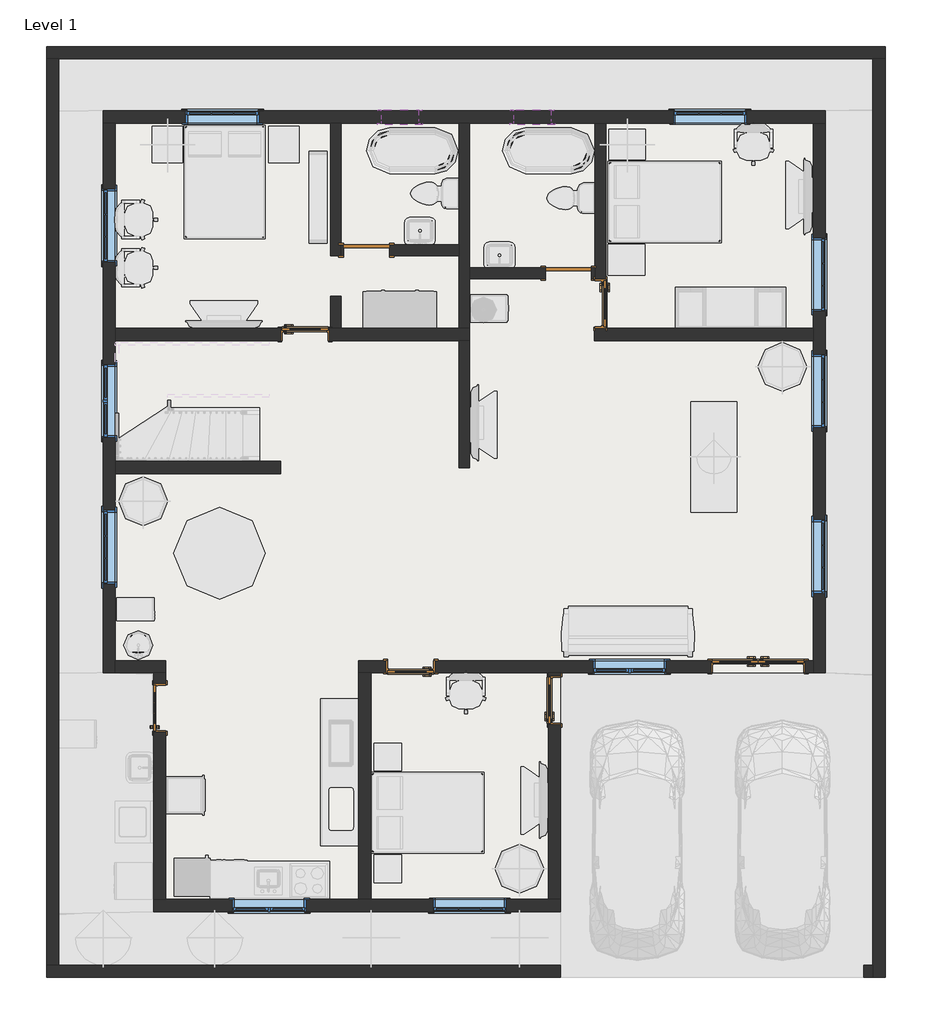
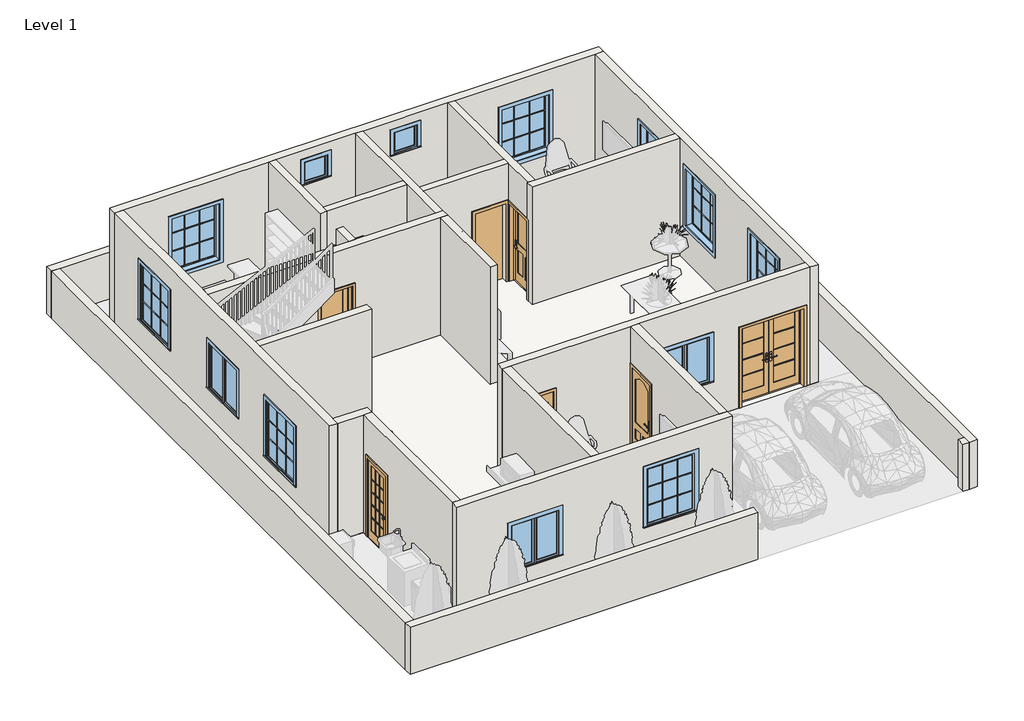
# One storey, part 1 of 3: 24 walls, 13 windows, 8 doors, 1 slab.
"""IFC4 building model written with IfcOpenShell, lengths in millimetres."""

from ifc_helpers import new_model, si_unit, frame, origin, origin_with_axes, place, context, project, spatial, polyline, outline, extrude, faceted_brep, transform, mapped, element, save
from components import door_41326d50, door_7e6851c9, door_3dfc5bb7, door_b03bd389, door_fe2643c7, door_ebd1a24e, door_41c6c2d7, window_cfa1ffdd, window_0862ab64, window_e41d21a6

model = new_model("IFC4")

# Units and contexts
model_context = context("Model", 3, world=origin())
ifc_project = project(units=[si_unit("LENGTHUNIT", "METRE", prefix="MILLI")], contexts=[model_context])

# Site, building, storey
site = spatial("IfcSite", under=ifc_project)
building = spatial("IfcBuilding", under=site)
storey = spatial("IfcBuildingStorey", under=building, Name="Level 1", Elevation=0.0)

# Doors
placement = place(None, origin())
door_shape = door_41326d50(model_context)
element("IfcDoor", 1, ObjectType="30\" x 80\"", at=placement, inside=storey, context=model_context, shape_type="MappedRepresentation", body=[
    mapped(door_shape, transform((-7358.6481534, 4188.5162111, 0.0), x_axis=(0.0, -1.0, 0.0), y_axis=(1.0, 0.0, 0.0), z_axis=(0.0, 0.0, 1.0))),
])
element("IfcDoor", 2, ObjectType="30\" x 80\"", at=placement, inside=storey, context=model_context, shape_type="MappedRepresentation", body=[
    mapped(door_shape, transform((-9743.0731534, 4744.1412111, 0.0), x_axis=(1.0, 0.0, 0.0), y_axis=(0.0, 1.0, 0.0), z_axis=(0.0, 0.0, 1.0))),
])
door_2_shape = door_7e6851c9(model_context)
element("IfcDoor", 3, ObjectType="30\" x 80\"", at=placement, inside=storey, context=model_context, shape_type="MappedRepresentation", body=[
    mapped(door_2_shape, transform((-11495.6731534, 10262.2912111, 0.0), x_axis=(-1.0, 0.0, 0.0), y_axis=(0.0, -1.0, 0.0), z_axis=(0.0, 0.0, 1.0))),
])
door_3_shape = door_3dfc5bb7(model_context)
element("IfcDoor", 4, ObjectType="30\" x 80\"", at=placement, inside=storey, context=model_context, shape_type="MappedRepresentation", body=[
    mapped(door_3_shape, transform((-6590.2981534, 10767.1162111, 0.0), x_axis=(0.0, 1.0, 0.0), y_axis=(-1.0, 0.0, 0.0), z_axis=(0.0, 0.0, 1.0))),
])
door_4_shape = door_b03bd389(model_context)
element("IfcDoor", 5, ObjectType="Door-Exterior-Double-Full Glass-Wood_Clad : 60\" x 80\"", at=placement, inside=storey, context=model_context, shape_type="MappedRepresentation", body=[
    mapped(door_4_shape, transform((-3977.2731534, 4750.4912111, 0.0), x_axis=(1.0, 0.0, 0.0), y_axis=(0.0, 1.0, 0.0), z_axis=(0.0, 0.0, 1.0))),
])
door_5_shape = door_fe2643c7(model_context)
element("IfcDoor", 6, ObjectType="Door-Interior-Single-Full Glass-Wood : 30\" x 80\"", at=placement, inside=storey, context=model_context, shape_type="MappedRepresentation", body=[
    mapped(door_5_shape, transform((-13911.8481534, 4061.5162111, 0.0), x_axis=(0.0, 1.0, 0.0), y_axis=(-1.0, 0.0, 0.0), z_axis=(0.0, 0.0, 1.0))),
])
door_6_shape = door_ebd1a24e(model_context)
element("IfcDoor", 7, ObjectType="Single-Flush : 30\" x 80\"", at=placement, inside=storey, context=model_context, shape_type="MappedRepresentation", body=[
    mapped(door_6_shape, transform((-10479.6731534, 11656.1162111, 0.0), x_axis=(-1.0, 0.0, 0.0), y_axis=(0.0, -1.0, 0.0), z_axis=(0.0, 0.0, 1.0))),
])
door_7_shape = door_41c6c2d7(model_context)
element("IfcDoor", 8, ObjectType="Single-Flush : 30\" x 80\"", at=placement, inside=storey, context=model_context, shape_type="MappedRepresentation", body=[
    mapped(door_7_shape, transform((-7126.8731534, 11275.1162111, 0.0), x_axis=(1.0, 0.0, 0.0), y_axis=(0.0, 1.0, 0.0), z_axis=(0.0, 0.0, 1.0))),
])

# Slab
element("IfcSlab", 9, at=placement, inside=storey, context=model_context, shape_type="SweptSolid", body=[
    extrude(outline(polyline([(-2859.6731534, 13967.5162111), (-2859.6731534, 4645.7162111), (-7253.8731534, 4645.7162111), (-7253.8731534, 683.3162111), (-14010.2731534, 683.3162111), (-14010.2731534, 4645.7162111), (-14848.4731534, 4645.7162111), (-14848.4731534, 13967.5162111), (-2859.6731534, 13967.5162111)])), frame((0.0, 0.0, -323.85), z_axis=(0.0, 0.0, 1.0), x_axis=(1.0, 0.0, 0.0)), (0.0, 0.0, 1.0), 323.85),
])

# Walls
element("IfcWall", 10, ObjectType="Generic - 8\"", at=placement, inside=storey, context=model_context, shape_type="SweptSolid", body=[
    extrude(outline(polyline([(-2224.6731534, -205.6837889), (-2072.2731534, -205.6837889), (-2072.2731534, -408.8837889), (-2224.6731534, -408.8837889), (-2224.6731534, -205.6837889)])), origin_with_axes(), (0.0, 0.0, 1.0), 1219.2),
])
element("IfcWall", 11, ObjectType="Generic - 8\"", at=placement, inside=storey, context=model_context, shape_type="Brep", body=[
    faceted_brep([(-14848.4731534, 13764.3162111, 0.0), (-14848.4731534, 4645.7162111, 0.0), (-14848.4731534, 4645.7162111, 3048.0), (-14848.4731534, 13764.3162111, 3048.0), (-14848.4731534, 7338.1162111, 2133.6), (-14848.4731534, 6118.9162111, 2133.6), (-14848.4731534, 6118.9162111, 609.6), (-14848.4731534, 7338.1162111, 609.6), (-14848.4731534, 12672.1162111, 2438.4), (-14848.4731534, 11452.9162111, 2438.4), (-14848.4731534, 11452.9162111, 914.4), (-14848.4731534, 12672.1162111, 914.4), (-14848.4731534, 9763.8162111, 2133.6), (-14848.4731534, 8544.6162111, 2133.6), (-14848.4731534, 8544.6162111, 914.4), (-14848.4731534, 9763.8162111, 914.4), (-14645.2731534, 13764.3162111, 0.0), (-14645.2731534, 13764.3162111, 3048.0), (-14645.2731534, 10360.7162111, 3048.0), (-14645.2731534, 10157.5162111, 3048.0), (-14645.2731534, 8150.9162111, 3048.0), (-14645.2731534, 7947.7162111, 3048.0), (-14645.2731534, 4848.9162111, 3048.0), (-14645.2731534, 4645.7162111, 3048.0), (-14645.2731534, 4645.7162111, 0.0), (-14645.2731534, 4848.9162111, 0.0), (-14645.2731534, 7947.7162111, 0.0), (-14645.2731534, 8150.9162111, 0.0), (-14645.2731534, 10157.5162111, 0.0), (-14645.2731534, 10360.7162111, 0.0), (-14645.2731534, 7338.1162111, 2133.6), (-14645.2731534, 7338.1162111, 609.6), (-14645.2731534, 6118.9162111, 609.6), (-14645.2731534, 6118.9162111, 2133.6), (-14645.2731534, 12672.1162111, 2438.4), (-14645.2731534, 12672.1162111, 914.4), (-14645.2731534, 11452.9162111, 914.4), (-14645.2731534, 11452.9162111, 2438.4), (-14645.2731534, 9763.8162111, 2133.6), (-14645.2731534, 9763.8162111, 914.4), (-14645.2731534, 8544.6162111, 914.4), (-14645.2731534, 8544.6162111, 2133.6)], [[[0, 1, 2, 3], [4, 5, 6, 7], [8, 9, 10, 11], [12, 13, 14, 15]], [[16, 17, 18, 19, 20, 21, 22, 23, 24, 25, 26, 27, 28, 29], [30, 31, 32, 33], [34, 35, 36, 37], [38, 39, 40, 41]], [[1, 0, 16, 29, 28, 27, 26, 25, 24]], [[3, 2, 23, 22, 21, 20, 19, 18, 17]], [[0, 3, 17, 16]], [[2, 1, 24, 23]], [[31, 30, 4, 7]], [[32, 31, 7, 6]], [[33, 32, 6, 5]], [[30, 33, 5, 4]], [[35, 34, 8, 11]], [[36, 35, 11, 10]], [[37, 36, 10, 9]], [[34, 37, 9, 8]], [[39, 38, 12, 15]], [[40, 39, 15, 14]], [[41, 40, 14, 13]], [[38, 41, 13, 12]]]),
])
element("IfcWall", 12, ObjectType="Generic - 8\"", at=placement, inside=storey, context=model_context, shape_type="Brep", body=[
    faceted_brep([(-3062.8731534, 13764.3162111, 0.0), (-3062.8731534, 10360.7162111, 0.0), (-3062.8731534, 10157.5162111, 0.0), (-3062.8731534, 4848.9162111, 0.0), (-3062.8731534, 4645.7162111, 0.0), (-3062.8731534, 4645.7162111, 3048.0), (-3062.8731534, 4848.9162111, 3048.0), (-3062.8731534, 10157.5162111, 3048.0), (-3062.8731534, 10360.7162111, 3048.0), (-3062.8731534, 13764.3162111, 3048.0), (-3062.8731534, 10640.1162111, 2438.4), (-3062.8731534, 10640.1162111, 914.4), (-3062.8731534, 11859.3162111, 914.4), (-3062.8731534, 11859.3162111, 2438.4), (-3062.8731534, 8709.7162111, 2438.4), (-3062.8731534, 8709.7162111, 914.4), (-3062.8731534, 9928.9162111, 914.4), (-3062.8731534, 9928.9162111, 2438.4), (-3062.8731534, 5966.5162111, 2438.4), (-3062.8731534, 5966.5162111, 914.4), (-3062.8731534, 7185.7162111, 914.4), (-3062.8731534, 7185.7162111, 2438.4), (-2859.6731534, 13764.3162111, 0.0), (-2859.6731534, 13764.3162111, 3048.0), (-2859.6731534, 4645.7162111, 3048.0), (-2859.6731534, 4645.7162111, 0.0), (-2859.6731534, 10640.1162111, 2438.4), (-2859.6731534, 11859.3162111, 2438.4), (-2859.6731534, 11859.3162111, 914.4), (-2859.6731534, 10640.1162111, 914.4), (-2859.6731534, 8709.7162111, 2438.4), (-2859.6731534, 9928.9162111, 2438.4), (-2859.6731534, 9928.9162111, 914.4), (-2859.6731534, 8709.7162111, 914.4), (-2859.6731534, 5966.5162111, 2438.4), (-2859.6731534, 7185.7162111, 2438.4), (-2859.6731534, 7185.7162111, 914.4), (-2859.6731534, 5966.5162111, 914.4)], [[[0, 1, 2, 3, 4, 5, 6, 7, 8, 9], [10, 11, 12, 13], [14, 15, 16, 17], [18, 19, 20, 21]], [[22, 23, 24, 25], [26, 27, 28, 29], [30, 31, 32, 33], [34, 35, 36, 37]], [[4, 3, 2, 1, 0, 22, 25]], [[9, 8, 7, 6, 5, 24, 23]], [[0, 9, 23, 22]], [[5, 4, 25, 24]], [[11, 10, 26, 29]], [[12, 11, 29, 28]], [[13, 12, 28, 27]], [[10, 13, 27, 26]], [[15, 14, 30, 33]], [[16, 15, 33, 32]], [[17, 16, 32, 31]], [[14, 17, 31, 30]], [[19, 18, 34, 37]], [[20, 19, 37, 36]], [[21, 20, 36, 35]], [[18, 21, 35, 34]]]),
])
element("IfcWall", 13, ObjectType="Generic - 8\"", at=placement, inside=storey, context=model_context, shape_type="Brep", body=[
    faceted_brep([(-2859.6731534, 13967.5162111, 0.0), (-14848.4731534, 13967.5162111, 0.0), (-14848.4731534, 13967.5162111, 3048.0), (-2859.6731534, 13967.5162111, 3048.0), (-12257.6731534, 13967.5162111, 2438.4), (-13476.8731534, 13967.5162111, 2438.4), (-13476.8731534, 13967.5162111, 914.4), (-12257.6731534, 13967.5162111, 914.4), (-4167.7731534, 13967.5162111, 2438.4), (-5386.9731534, 13967.5162111, 2438.4), (-5386.9731534, 13967.5162111, 914.4), (-4167.7731534, 13967.5162111, 914.4), (-10225.6731534, 13967.5162111, 2768.6), (-10225.6731534, 13967.5162111, 2159.0), (-9616.0731534, 13967.5162111, 2159.0), (-9616.0731534, 13967.5162111, 2768.6), (-8028.5731534, 13967.5162111, 2768.6), (-8028.5731534, 13967.5162111, 2159.0), (-7418.9731534, 13967.5162111, 2159.0), (-7418.9731534, 13967.5162111, 2768.6), (-2859.6731534, 13764.3162111, 0.0), (-2859.6731534, 13764.3162111, 3048.0), (-3062.8731534, 13764.3162111, 3048.0), (-6504.5731534, 13764.3162111, 3048.0), (-6682.3731534, 13764.3162111, 3048.0), (-8765.1731534, 13764.3162111, 3048.0), (-8942.9731534, 13764.3162111, 3048.0), (-10898.7731534, 13764.3162111, 3048.0), (-11076.5731534, 13764.3162111, 3048.0), (-14645.2731534, 13764.3162111, 3048.0), (-14848.4731534, 13764.3162111, 3048.0), (-14848.4731534, 13764.3162111, 0.0), (-14645.2731534, 13764.3162111, 0.0), (-11076.5731534, 13764.3162111, 0.0), (-10898.7731534, 13764.3162111, 0.0), (-8942.9731534, 13764.3162111, 0.0), (-8765.1731534, 13764.3162111, 0.0), (-6682.3731534, 13764.3162111, 0.0), (-6504.5731534, 13764.3162111, 0.0), (-3062.8731534, 13764.3162111, 0.0), (-12257.6731534, 13764.3162111, 2438.4), (-12257.6731534, 13764.3162111, 914.4), (-13476.8731534, 13764.3162111, 914.4), (-13476.8731534, 13764.3162111, 2438.4), (-4167.7731534, 13764.3162111, 2438.4), (-4167.7731534, 13764.3162111, 914.4), (-5386.9731534, 13764.3162111, 914.4), (-5386.9731534, 13764.3162111, 2438.4), (-10225.6731534, 13764.3162111, 2768.6), (-9616.0731534, 13764.3162111, 2768.6), (-9616.0731534, 13764.3162111, 2159.0), (-10225.6731534, 13764.3162111, 2159.0), (-8028.5731534, 13764.3162111, 2768.6), (-7418.9731534, 13764.3162111, 2768.6), (-7418.9731534, 13764.3162111, 2159.0), (-8028.5731534, 13764.3162111, 2159.0)], [[[0, 1, 2, 3], [4, 5, 6, 7], [8, 9, 10, 11], [12, 13, 14, 15], [16, 17, 18, 19]], [[20, 21, 22, 23, 24, 25, 26, 27, 28, 29, 30, 31, 32, 33, 34, 35, 36, 37, 38, 39], [40, 41, 42, 43], [44, 45, 46, 47], [48, 49, 50, 51], [52, 53, 54, 55]], [[1, 0, 20, 39, 38, 37, 36, 35, 34, 33, 32, 31]], [[3, 2, 30, 29, 28, 27, 26, 25, 24, 23, 22, 21]], [[2, 1, 31, 30]], [[0, 3, 21, 20]], [[41, 40, 4, 7]], [[42, 41, 7, 6]], [[43, 42, 6, 5]], [[40, 43, 5, 4]], [[45, 44, 8, 11]], [[46, 45, 11, 10]], [[47, 46, 10, 9]], [[44, 47, 9, 8]], [[13, 12, 48, 51]], [[14, 13, 51, 50]], [[15, 14, 50, 49]], [[12, 15, 49, 48]], [[17, 16, 52, 55]], [[18, 17, 55, 54]], [[19, 18, 54, 53]], [[16, 19, 53, 52]]]),
])
element("IfcWall", 14, ObjectType="Generic - 8\"", at=placement, inside=storey, context=model_context, shape_type="Brep", body=[
    faceted_brep([(-14645.2731534, 4645.7162111, 0.0), (-14010.2731534, 4645.7162111, 0.0), (-13807.0731534, 4645.7162111, 0.0), (-13807.0731534, 4645.7162111, 3048.0), (-14010.2731534, 4645.7162111, 3048.0), (-14645.2731534, 4645.7162111, 3048.0), (-14645.2731534, 4848.9162111, 0.0), (-14645.2731534, 4848.9162111, 3048.0), (-13807.0731534, 4848.9162111, 3048.0), (-13807.0731534, 4848.9162111, 0.0)], [[[0, 1, 2, 3, 4, 5]], [[6, 7, 8, 9]], [[2, 1, 0, 6, 9]], [[3, 2, 9, 8]], [[5, 4, 3, 8, 7]], [[0, 5, 7, 6]]]),
])
element("IfcWall", 15, ObjectType="Generic - 8\"", at=placement, inside=storey, context=model_context, shape_type="SweptSolid", body=[
    extrude(outline(polyline([(-10606.6731534, 886.5162111), (-10606.6731534, 4645.7162111), (-10403.4731534, 4645.7162111), (-10403.4731534, 886.5162111), (-10606.6731534, 886.5162111)])), origin_with_axes(), (0.0, 0.0, 1.0), 3048.0),
])
element("IfcWall", 16, ObjectType="Generic - 8\"", at=placement, inside=storey, context=model_context, shape_type="SweptSolid", body=[
    extrude(outline(polyline([(886.5162111, 3048.0), (4645.7162111, 3048.0), (4645.7162111, 0.0), (4467.9162111, 0.0), (4467.9162111, 2057.4), (3655.1162111, 2057.4), (3655.1162111, 0.0), (886.5162111, 0.0), (886.5162111, 3048.0)])), frame((-14010.2731534, 0.0, 0.0), z_axis=(1.0, 0.0, 0.0), x_axis=(0.0, 1.0, 0.0)), (0.0, 0.0, 1.0), 203.2),
])
element("IfcWall", 17, ObjectType="Generic - 8\"", at=placement, inside=storey, context=model_context, shape_type="Brep", body=[
    faceted_brep([(-14010.2731534, 683.3162111, 0.0), (-7253.8731534, 683.3162111, 0.0), (-7253.8731534, 683.3162111, 3048.0), (-14010.2731534, 683.3162111, 3048.0), (-9374.7731534, 683.3162111, 2438.4), (-8155.5731534, 683.3162111, 2438.4), (-8155.5731534, 683.3162111, 914.4), (-9374.7731534, 683.3162111, 914.4), (-12702.1731534, 683.3162111, 2133.6), (-11482.9731534, 683.3162111, 2133.6), (-11482.9731534, 683.3162111, 914.4), (-12702.1731534, 683.3162111, 914.4), (-14010.2731534, 886.5162111, 0.0), (-14010.2731534, 886.5162111, 3048.0), (-13807.0731534, 886.5162111, 3048.0), (-10606.6731534, 886.5162111, 3048.0), (-10403.4731534, 886.5162111, 3048.0), (-7457.0731534, 886.5162111, 3048.0), (-7253.8731534, 886.5162111, 3048.0), (-7253.8731534, 886.5162111, 0.0), (-7457.0731534, 886.5162111, 0.0), (-10403.4731534, 886.5162111, 0.0), (-10606.6731534, 886.5162111, 0.0), (-13807.0731534, 886.5162111, 0.0), (-9374.7731534, 886.5162111, 2438.4), (-9374.7731534, 886.5162111, 914.4), (-8155.5731534, 886.5162111, 914.4), (-8155.5731534, 886.5162111, 2438.4), (-12702.1731534, 886.5162111, 2133.6), (-12702.1731534, 886.5162111, 914.4), (-11482.9731534, 886.5162111, 914.4), (-11482.9731534, 886.5162111, 2133.6)], [[[0, 1, 2, 3], [4, 5, 6, 7], [8, 9, 10, 11]], [[12, 13, 14, 15, 16, 17, 18, 19, 20, 21, 22, 23], [24, 25, 26, 27], [28, 29, 30, 31]], [[1, 0, 12, 23, 22, 21, 20, 19]], [[3, 2, 18, 17, 16, 15, 14, 13]], [[0, 3, 13, 12]], [[2, 1, 19, 18]], [[25, 24, 4, 7]], [[26, 25, 7, 6]], [[27, 26, 6, 5]], [[24, 27, 5, 4]], [[29, 28, 8, 11]], [[30, 29, 11, 10]], [[31, 30, 10, 9]], [[28, 31, 9, 8]]]),
])
element("IfcWall", 18, ObjectType="Generic - 8\"", at=placement, inside=storey, context=model_context, shape_type="SweptSolid", body=[
    extrude(outline(polyline([(886.5162111, 3048.0), (4645.7162111, 3048.0), (4645.7162111, 0.0), (4594.9162111, 0.0), (4594.9162111, 2057.4), (3782.1162111, 2057.4), (3782.1162111, 0.0), (886.5162111, 0.0), (886.5162111, 3048.0)])), frame((-7457.0731534, 0.0, 0.0), z_axis=(1.0, 0.0, 0.0), x_axis=(0.0, 1.0, 0.0)), (0.0, 0.0, 1.0), 203.2),
])
element("IfcWall", 19, ObjectType="Generic - 8\"", at=placement, inside=storey, context=model_context, shape_type="Brep", body=[
    faceted_brep([(-8765.1731534, 10157.5162111, 3048.0), (-8942.9731534, 10157.5162111, 3048.0), (-14645.2731534, 10157.5162111, 3048.0), (-14645.2731534, 10157.5162111, 0.0), (-11902.0731534, 10157.5162111, 0.0), (-11902.0731534, 10157.5162111, 2057.4), (-11089.2731534, 10157.5162111, 2057.4), (-11089.2731534, 10157.5162111, 0.0), (-8942.9731534, 10157.5162111, 0.0), (-8765.1731534, 10157.5162111, 0.0), (-14645.2731534, 10360.7162111, 3048.0), (-11076.5731534, 10360.7162111, 3048.0), (-10898.7731534, 10360.7162111, 3048.0), (-8942.9731534, 10360.7162111, 3048.0), (-8765.1731534, 10360.7162111, 3048.0), (-8765.1731534, 10360.7162111, 0.0), (-8942.9731534, 10360.7162111, 0.0), (-10898.7731534, 10360.7162111, 0.0), (-11076.5731534, 10360.7162111, 0.0), (-11089.2731534, 10360.7162111, 0.0), (-11089.2731534, 10360.7162111, 2057.4), (-11902.0731534, 10360.7162111, 2057.4), (-11902.0731534, 10360.7162111, 0.0), (-14645.2731534, 10360.7162111, 0.0)], [[[0, 1, 2, 3, 4, 5, 6, 7, 8, 9]], [[10, 11, 12, 13, 14, 15, 16, 17, 18, 19, 20, 21, 22, 23]], [[3, 23, 22, 4]], [[15, 9, 8, 7, 19, 18, 17, 16]], [[2, 1, 0, 14, 13, 12, 11, 10]], [[3, 2, 10, 23]], [[0, 9, 15, 14]], [[21, 5, 4, 22]], [[5, 21, 20, 6]], [[6, 20, 19, 7]]]),
])
element("IfcWall", 20, ObjectType="Generic - 8\"", at=placement, inside=storey, context=model_context, shape_type="Brep", body=[
    faceted_brep([(-6695.0731534, 10157.5162111, 0.0), (-3062.8731534, 10157.5162111, 0.0), (-3062.8731534, 10157.5162111, 3048.0), (-6695.0731534, 10157.5162111, 3048.0), (-6695.0731534, 10360.7162111, 0.0), (-6695.0731534, 10360.7162111, 3048.0), (-6682.3731534, 10360.7162111, 3048.0), (-6504.5731534, 10360.7162111, 3048.0), (-3062.8731534, 10360.7162111, 3048.0), (-3062.8731534, 10360.7162111, 0.0)], [[[0, 1, 2, 3]], [[4, 5, 6, 7, 8, 9]], [[1, 0, 4, 9]], [[3, 2, 8, 7, 6, 5]], [[0, 3, 5, 4]], [[2, 1, 9, 8]]]),
])
element("IfcWall", 21, ObjectType="Generic - 8\"", at=placement, inside=storey, context=model_context, shape_type="SweptSolid", body=[
    extrude(outline(polyline([(-11902.0731534, 7947.7162111), (-14645.2731534, 7947.7162111), (-14645.2731534, 8150.9162111), (-11902.0731534, 8150.9162111), (-11902.0731534, 7947.7162111)])), origin_with_axes(), (0.0, 0.0, 1.0), 3048.0),
])
element("IfcWall", 22, ObjectType="Generic - 8\"", at=placement, inside=storey, context=model_context, shape_type="Brep", body=[
    faceted_brep([(-3062.8731534, 4645.7162111, 3048.0), (-7253.8731534, 4645.7162111, 3048.0), (-7457.0731534, 4645.7162111, 3048.0), (-10403.4731534, 4645.7162111, 3048.0), (-10606.6731534, 4645.7162111, 3048.0), (-10606.6731534, 4645.7162111, 0.0), (-10403.4731534, 4645.7162111, 0.0), (-10149.4731534, 4645.7162111, 0.0), (-10149.4731534, 4645.7162111, 2057.4), (-9336.6731534, 4645.7162111, 2057.4), (-9336.6731534, 4645.7162111, 0.0), (-7457.0731534, 4645.7162111, 0.0), (-7253.8731534, 4645.7162111, 0.0), (-4764.6731534, 4645.7162111, 0.0), (-4764.6731534, 4645.7162111, 2057.4), (-3189.8731534, 4645.7162111, 2057.4), (-3189.8731534, 4645.7162111, 0.0), (-3062.8731534, 4645.7162111, 0.0), (-6720.4731534, 4645.7162111, 2133.6), (-5501.2731534, 4645.7162111, 2133.6), (-5501.2731534, 4645.7162111, 914.4), (-6720.4731534, 4645.7162111, 914.4), (-10606.6731534, 4848.9162111, 3048.0), (-3062.8731534, 4848.9162111, 3048.0), (-3062.8731534, 4848.9162111, 0.0), (-3189.8731534, 4848.9162111, 0.0), (-3189.8731534, 4848.9162111, 2057.4), (-4764.6731534, 4848.9162111, 2057.4), (-4764.6731534, 4848.9162111, 0.0), (-9336.6731534, 4848.9162111, 0.0), (-9336.6731534, 4848.9162111, 2057.4), (-10149.4731534, 4848.9162111, 2057.4), (-10149.4731534, 4848.9162111, 0.0), (-10606.6731534, 4848.9162111, 0.0), (-6720.4731534, 4848.9162111, 2133.6), (-6720.4731534, 4848.9162111, 914.4), (-5501.2731534, 4848.9162111, 914.4), (-5501.2731534, 4848.9162111, 2133.6)], [[[0, 1, 2, 3, 4, 5, 6, 7, 8, 9, 10, 11, 12, 13, 14, 15, 16, 17], [18, 19, 20, 21]], [[22, 23, 24, 25, 26, 27, 28, 29, 30, 31, 32, 33], [34, 35, 36, 37]], [[24, 17, 16, 25]], [[5, 33, 32, 7, 6]], [[28, 13, 12, 11, 10, 29]], [[4, 3, 2, 1, 0, 23, 22]], [[0, 17, 24, 23]], [[5, 4, 22, 33]], [[15, 26, 25, 16]], [[26, 15, 14, 27]], [[27, 14, 13, 28]], [[9, 30, 29, 10]], [[30, 9, 8, 31]], [[31, 8, 7, 32]], [[35, 34, 18, 21]], [[36, 35, 21, 20]], [[37, 36, 20, 19]], [[34, 37, 19, 18]]]),
])
element("IfcWall", 23, ObjectType="INNER WALL", at=placement, inside=storey, context=model_context, shape_type="Brep", body=[
    faceted_brep([(-11076.5731534, 13764.3162111, 0.0), (-11076.5731534, 11567.2162111, 0.0), (-11076.5731534, 11567.2162111, 3048.0), (-11076.5731534, 13764.3162111, 3048.0), (-10898.7731534, 13764.3162111, 0.0), (-10898.7731534, 13764.3162111, 3048.0), (-10898.7731534, 11745.0162111, 3048.0), (-10898.7731534, 11567.2162111, 3048.0), (-10898.7731534, 11567.2162111, 0.0), (-10898.7731534, 11745.0162111, 0.0)], [[[0, 1, 2, 3]], [[4, 5, 6, 7, 8, 9]], [[1, 0, 4, 9, 8]], [[3, 2, 7, 6, 5]], [[0, 3, 5, 4]], [[2, 1, 8, 7]]]),
])
element("IfcWall", 24, ObjectType="INNER WALL", at=placement, inside=storey, context=model_context, shape_type="Brep", body=[
    faceted_brep([(-6504.5731534, 13764.3162111, 3048.0), (-6504.5731534, 10360.7162111, 3048.0), (-6504.5731534, 10360.7162111, 2057.4), (-6504.5731534, 11173.5162111, 2057.4), (-6504.5731534, 11173.5162111, 0.0), (-6504.5731534, 13764.3162111, 0.0), (-6682.3731534, 10360.7162111, 3048.0), (-6682.3731534, 11186.2162111, 3048.0), (-6682.3731534, 11364.0162111, 3048.0), (-6682.3731534, 13764.3162111, 3048.0), (-6682.3731534, 13764.3162111, 0.0), (-6682.3731534, 11364.0162111, 0.0), (-6682.3731534, 11186.2162111, 0.0), (-6682.3731534, 11173.5162111, 0.0), (-6682.3731534, 11173.5162111, 2057.4), (-6682.3731534, 10360.7162111, 2057.4)], [[[0, 1, 2, 3, 4, 5]], [[6, 7, 8, 9, 10, 11, 12, 13, 14, 15]], [[10, 5, 4, 13, 12, 11]], [[1, 0, 9, 8, 7, 6]], [[0, 5, 10, 9]], [[1, 6, 15, 2]], [[3, 14, 13, 4]], [[14, 3, 2, 15]]]),
])
element("IfcWall", 25, ObjectType="INNER WALL", at=placement, inside=storey, context=model_context, shape_type="Brep", body=[
    faceted_brep([(-8942.9731534, 13764.3162111, 0.0), (-8942.9731534, 11745.0162111, 0.0), (-8942.9731534, 11567.2162111, 0.0), (-8942.9731534, 10360.7162111, 0.0), (-8942.9731534, 10360.7162111, 3048.0), (-8942.9731534, 11567.2162111, 3048.0), (-8942.9731534, 11745.0162111, 3048.0), (-8942.9731534, 13764.3162111, 3048.0), (-8765.1731534, 13764.3162111, 0.0), (-8765.1731534, 13764.3162111, 3048.0), (-8765.1731534, 11364.0162111, 3048.0), (-8765.1731534, 11186.2162111, 3048.0), (-8765.1731534, 10360.7162111, 3048.0), (-8765.1731534, 10360.7162111, 0.0), (-8765.1731534, 11186.2162111, 0.0), (-8765.1731534, 11364.0162111, 0.0)], [[[0, 1, 2, 3, 4, 5, 6, 7]], [[8, 9, 10, 11, 12, 13, 14, 15]], [[3, 2, 1, 0, 8, 15, 14, 13]], [[7, 6, 5, 4, 12, 11, 10, 9]], [[0, 7, 9, 8]], [[4, 3, 13, 12]]]),
])
element("IfcWall", 26, ObjectType="INNER WALL", at=placement, inside=storey, context=model_context, shape_type="SweptSolid", body=[
    extrude(outline(polyline([(0.0, -10898.7731534), (0.0, -10860.6731534), (2032.0, -10860.6731534), (2032.0, -10098.6731534), (0.0, -10098.6731534), (0.0, -8942.9731534), (3048.0, -8942.9731534), (3048.0, -10898.7731534), (0.0, -10898.7731534)])), frame((0.0, 11567.2162111, 0.0), z_axis=(0.0, 1.0, 0.0), x_axis=(0.0, 0.0, 1.0)), (0.0, 0.0, 1.0), 177.8),
])
element("IfcWall", 27, ObjectType="INNER WALL", at=placement, inside=storey, context=model_context, shape_type="SweptSolid", body=[
    extrude(outline(polyline([(2032.0, -6745.8731534), (0.0, -6745.8731534), (0.0, -6682.3731534), (3048.0, -6682.3731534), (3048.0, -8765.1731534), (0.0, -8765.1731534), (0.0, -7507.8731534), (2032.0, -7507.8731534), (2032.0, -6745.8731534)])), frame((0.0, 11186.2162111, 0.0), z_axis=(0.0, 1.0, 0.0), x_axis=(0.0, 0.0, 1.0)), (0.0, 0.0, 1.0), 177.8),
])
element("IfcWall", 28, ObjectType="INNER WALL", at=placement, inside=storey, context=model_context, shape_type="SweptSolid", body=[
    extrude(outline(polyline([(-11076.5731534, 10360.7162111), (-11076.5731534, 10894.1162111), (-10898.7731534, 10894.1162111), (-10898.7731534, 10360.7162111), (-11076.5731534, 10360.7162111)])), origin_with_axes(), (0.0, 0.0, 1.0), 3048.0),
])
element("IfcWall", 29, ObjectType="INNER WALL", at=placement, inside=storey, context=model_context, shape_type="SweptSolid", body=[
    extrude(outline(polyline([(-8942.9731534, 8049.3162111), (-8942.9731534, 10157.5162111), (-8765.1731534, 10157.5162111), (-8765.1731534, 8049.3162111), (-8942.9731534, 8049.3162111)])), origin_with_axes(), (0.0, 0.0, 1.0), 3048.0),
])
element("IfcWall", 30, ObjectType="OUTER WALL", at=placement, inside=storey, context=model_context, shape_type="Brep", body=[
    faceted_brep([(-15788.2731534, 14831.1162111, 0.0), (-15585.0731534, 14831.1162111, 0.0), (-2072.2731534, 14831.1162111, 0.0), (-1869.0731534, 14831.1162111, 0.0), (-1869.0731534, 14831.1162111, 1219.2), (-2072.2731534, 14831.1162111, 1219.2), (-15585.0731534, 14831.1162111, 1219.2), (-15788.2731534, 14831.1162111, 1219.2), (-15788.2731534, 15034.3162111, 0.0), (-15788.2731534, 15034.3162111, 1219.2), (-1869.0731534, 15034.3162111, 1219.2), (-1869.0731534, 15034.3162111, 0.0)], [[[0, 1, 2, 3, 4, 5, 6, 7]], [[8, 9, 10, 11]], [[3, 2, 1, 0, 8, 11]], [[7, 6, 5, 4, 10, 9]], [[4, 3, 11, 10]], [[0, 7, 9, 8]]]),
])
element("IfcWall", 31, ObjectType="OUTER WALL", at=placement, inside=storey, context=model_context, shape_type="Brep", body=[
    faceted_brep([(-2072.2731534, 14831.1162111, 0.0), (-2072.2731534, -205.6837889, 0.0), (-2072.2731534, -408.8837889, 0.0), (-2072.2731534, -408.8837889, 1219.2), (-2072.2731534, -205.6837889, 1219.2), (-2072.2731534, 14831.1162111, 1219.2), (-1869.0731534, 14831.1162111, 0.0), (-1869.0731534, 14831.1162111, 1219.2), (-1869.0731534, -408.8837889, 1219.2), (-1869.0731534, -408.8837889, 0.0)], [[[0, 1, 2, 3, 4, 5]], [[6, 7, 8, 9]], [[2, 1, 0, 6, 9]], [[5, 4, 3, 8, 7]], [[0, 5, 7, 6]], [[3, 2, 9, 8]]]),
])
element("IfcWall", 32, ObjectType="OUTER WALL", at=placement, inside=storey, context=model_context, shape_type="SweptSolid", body=[
    extrude(outline(polyline([(-15585.0731534, 14831.1162111), (-15585.0731534, -205.6837889), (-15788.2731534, -205.6837889), (-15788.2731534, 14831.1162111), (-15585.0731534, 14831.1162111)])), origin_with_axes(), (0.0, 0.0, 1.0), 1219.2),
])
element("IfcWall", 33, ObjectType="OUTER WALL", at=placement, inside=storey, context=model_context, shape_type="Brep", body=[
    faceted_brep([(-7253.8731534, -205.6837889, 0.0), (-15585.0731534, -205.6837889, 0.0), (-15788.2731534, -205.6837889, 0.0), (-15788.2731534, -205.6837889, 1219.2), (-15585.0731534, -205.6837889, 1219.2), (-7253.8731534, -205.6837889, 1219.2), (-7253.8731534, -408.8837889, 0.0), (-7253.8731534, -408.8837889, 1219.2), (-15788.2731534, -408.8837889, 1219.2), (-15788.2731534, -408.8837889, 0.0)], [[[0, 1, 2, 3, 4, 5]], [[6, 7, 8, 9]], [[2, 1, 0, 6, 9]], [[5, 4, 3, 8, 7]], [[0, 5, 7, 6]], [[3, 2, 9, 8]]]),
])

# Windows
window_shape = window_cfa1ffdd(model_context)
element("IfcWindow", 34, ObjectType="Casement 3x3 with Trim : 48\" x 60\"", at=placement, inside=storey, context=model_context, shape_type="MappedRepresentation", body=[
    mapped(window_shape, transform((-8765.1731534, 784.9162111, 304.8), x_axis=(-1.0, 0.0, 0.0), y_axis=(0.0, -1.0, 0.0), z_axis=(0.0, 0.0, 1.0))),
])
element("IfcWindow", 35, ObjectType="Casement 3x3 with Trim : 48\" x 60\"", at=placement, inside=storey, context=model_context, shape_type="MappedRepresentation", body=[
    mapped(window_shape, transform((-14746.8731534, 6728.5162111, 0.0), x_axis=(0.0, 1.0, 0.0), y_axis=(-1.0, 0.0, 0.0), z_axis=(0.0, 0.0, 1.0))),
])
element("IfcWindow", 36, ObjectType="Casement 3x3 with Trim : 48\" x 60\"", at=placement, inside=storey, context=model_context, shape_type="MappedRepresentation", body=[
    mapped(window_shape, transform((-14746.8731534, 12062.5162111, 304.8), x_axis=(0.0, 1.0, 0.0), y_axis=(-1.0, 0.0, 0.0), z_axis=(0.0, 0.0, 1.0))),
])
element("IfcWindow", 37, ObjectType="Casement 3x3 with Trim : 48\" x 60\"", at=placement, inside=storey, context=model_context, shape_type="MappedRepresentation", body=[
    mapped(window_shape, transform((-12867.2731534, 13865.9162111, 304.8), x_axis=(1.0, 0.0, 0.0), y_axis=(0.0, 1.0, 0.0), z_axis=(0.0, 0.0, 1.0))),
])
element("IfcWindow", 38, ObjectType="Casement 3x3 with Trim : 48\" x 60\"", at=placement, inside=storey, context=model_context, shape_type="MappedRepresentation", body=[
    mapped(window_shape, transform((-4777.3731534, 13865.9162111, 304.8), x_axis=(1.0, 0.0, 0.0), y_axis=(0.0, 1.0, 0.0), z_axis=(0.0, 0.0, 1.0))),
])
element("IfcWindow", 39, ObjectType="Casement 3x3 with Trim : 48\" x 60\"", at=placement, inside=storey, context=model_context, shape_type="MappedRepresentation", body=[
    mapped(window_shape, transform((-2961.2731534, 11249.7162111, 304.8), x_axis=(0.0, -1.0, 0.0), y_axis=(1.0, 0.0, 0.0), z_axis=(0.0, 0.0, 1.0))),
])
element("IfcWindow", 40, ObjectType="Casement 3x3 with Trim : 48\" x 60\"", at=placement, inside=storey, context=model_context, shape_type="MappedRepresentation", body=[
    mapped(window_shape, transform((-2961.2731534, 9319.3162111, 304.8), x_axis=(0.0, -1.0, 0.0), y_axis=(1.0, 0.0, 0.0), z_axis=(0.0, 0.0, 1.0))),
])
element("IfcWindow", 41, ObjectType="Casement 3x3 with Trim : 48\" x 60\"", at=placement, inside=storey, context=model_context, shape_type="MappedRepresentation", body=[
    mapped(window_shape, transform((-2961.2731534, 6576.1162111, 304.8), x_axis=(0.0, -1.0, 0.0), y_axis=(1.0, 0.0, 0.0), z_axis=(0.0, 0.0, 1.0))),
])
window_2_shape = window_0862ab64(model_context)
element("IfcWindow", 42, ObjectType="Casement Dbl with Trim : 48\" x 48\"", at=placement, inside=storey, context=model_context, shape_type="MappedRepresentation", body=[
    mapped(window_2_shape, transform((-12092.5731534, 803.9662111, 0.0), x_axis=(-1.0, 0.0, 0.0), y_axis=(0.0, -1.0, 0.0), z_axis=(0.0, 0.0, 1.0))),
])
element("IfcWindow", 43, ObjectType="Casement Dbl with Trim : 48\" x 48\"", at=placement, inside=storey, context=model_context, shape_type="MappedRepresentation", body=[
    mapped(window_2_shape, transform((-6110.8731534, 4766.3662111, 0.0), x_axis=(-1.0, 0.0, 0.0), y_axis=(0.0, -1.0, 0.0), z_axis=(0.0, 0.0, 1.0))),
])
element("IfcWindow", 44, ObjectType="Casement Dbl with Trim : 48\" x 48\"", at=placement, inside=storey, context=model_context, shape_type="MappedRepresentation", body=[
    mapped(window_2_shape, transform((-14727.8231534, 9154.2162111, 0.0), x_axis=(0.0, 1.0, 0.0), y_axis=(-1.0, 0.0, 0.0), z_axis=(0.0, 0.0, 1.0))),
])
window_3_shape = window_e41d21a6(model_context)
element("IfcWindow", 45, ObjectType="Transom with Trim : 24\" x 24\"", at=placement, inside=storey, context=model_context, shape_type="MappedRepresentation", body=[
    mapped(window_3_shape, transform((-9958.9731534, 13865.9162111, 0.0), x_axis=(-1.0, 0.0, 0.0), y_axis=(0.0, -1.0, 0.0), z_axis=(0.0, 0.0, 1.0))),
])
element("IfcWindow", 46, ObjectType="Transom with Trim : 24\" x 24\"", at=placement, inside=storey, context=model_context, shape_type="MappedRepresentation", body=[
    mapped(window_3_shape, transform((-7761.8731534, 13865.9162111, 0.0), x_axis=(-1.0, 0.0, 0.0), y_axis=(0.0, -1.0, 0.0), z_axis=(0.0, 0.0, 1.0))),
])

save(model, "model.ifc")

# Revit data of these elements
# Type "30\" x 80\""
#   Type Mark = "9"
#   Assembly Code = "B2030100"
#   Analytic Construction = "French door, wood frame with single glass"
#   Threshold Offset [instance default] = 0' - 0 1/2"
#   Thickness = 0' - 1 3/8"
#   Thermal Resistance (R) = 1.0696 (h·ft²·°F)/BTU
#   Swing Angle [instance default] = 90.00°
#   Stiles = 0' - 4 3/4"
#   Rough Width = 2' - 8"
#   Rough Height = 6' - 9"
#   Radius = 1' - 1.00625"
#   Lock Rail = 0' - 7 1/8"
#   Height = 6' - 8"
#   Width = 2' - 6"
#   Heat Transfer Coefficient (U) = 0.9350 BTU/(h·ft²·°F)
#   Door Offset [instance default] = 0' - 0"
#   Bottom Rail = 0' - 9 1/2"
#   Threshold [instance default] = yes
#   Function = 1
#   Exterior Trim [instance default] = yes
#   Trim Material = Cherry
#   Threshold Material = Cherry
#   Panel Material = Cherry
#   Glazing = Glass
#   Frame Material = Cherry
#   Door Handle Material = Aluminum
#   Visual Light Transmittance = 0
#   Solar Heat Gain Coefficient = 0
#   Wall Closure = (empty or 0)
#   Construction Type = (empty or 0)
# Type "30\" x 80\""
#   Type Mark = "10"
#   Assembly Code = "B2030100"
#   Analytic Construction = "French door, wood frame with single glass"
#   Top Rail = 0' - 4 3/4"
#   Threshold Offset [instance default] = 0' - 0 1/2"
#   Thickness = 0' - 1 3/8"
#   Thermal Resistance (R) = 1.0696 (h·ft²·°F)/BTU
#   Swing Angle [instance default] = 90.00°
#   Stiles = 0' - 4 3/4"
#   Rough Width = 2' - 8"
#   Rough Height = 6' - 9"
#   Lock Rail = 0' - 7 1/8"
#   Height = 6' - 8"
#   Width = 2' - 6"
#   Heat Transfer Coefficient (U) = 0.9350 BTU/(h·ft²·°F)
#   Door Offset [instance default] = 0' - 0"
#   Bottom Rail = 0' - 9 1/2"
#   Threshold [instance default] = yes
#   Function = 1
#   Exterior Trim [instance default] = yes
#   Trim Material = Cherry
#   Threshold Material = Cherry
#   Panel Material = Cherry
#   Glazing = Glass
#   Frame Material = Cherry
#   Door Handle Material = Aluminum
#   Visual Light Transmittance = 0
#   Solar Heat Gain Coefficient = 0
#   Wall Closure = (empty or 0)
#   Construction Type = (empty or 0)
# Type "Door-Exterior-Double-Full Glass-Wood_Clad : 60\" x 80\""
#   Type Mark = "8"
#   Assembly Code = "B2030100"
#   Analytic Construction = "French door, wood frame with double glass"
#   Top Rail = 0' - 4 11/16"
#   Threshold Offset [instance default] = 0' - 0 1/2"
#   Thickness = 0' - 1 3/8"
#   Thermal Resistance (R) = 1.9158 (h·ft²·°F)/BTU
#   Swing Angle [instance default] = 90.00°
#   Stiles = 0' - 4 3/4"
#   Rough Width = 5' - 2"
#   Rough Height = 6' - 9"
#   Panel Width = 2' - 6"
#   Door Offset [instance default] = 0' - 0"
#   Height = 6' - 8"
#   Width = 5' - 0"
#   Heat Transfer Coefficient (U) = 0.5220 BTU/(h·ft²·°F)
#   Bottom Rail = 0' - 9 1/8"
#   Exterior Trim [instance default] = yes
#   Threshold [instance default] = yes
#   Show Grill [instance default] = yes
#   Function = 1
#   Trim Material = Cherry
#   Threshold Material = Cherry
#   Panel Material = Cherry
#   Glazing = Glass
#   Frame Material = Cherry
#   Door Handle Material = Aluminum
#   Visual Light Transmittance = 0
#   Solar Heat Gain Coefficient = 0
#   Wall Closure = (empty or 0)
#   Construction Type = (empty or 0)
# Type "Door-Interior-Single-Full Glass-Wood : 30\" x 80\""
#   Type Mark = "11"
#   Assembly Code = "C1020300"
#   Analytic Construction = "Wood frame with single clear glass"
#   Top Rail = 0' - 4 11/16"
#   Thickness = 0' - 1 3/8"
#   Thermal Resistance (R) = 1.0102 (h·ft²·°F)/BTU
#   Swing Angle [instance default] = 90.00°
#   Stiles = 0' - 4 3/4"
#   Rough Width = 2' - 8"
#   Rough Height = 6' - 9"
#   Height = 6' - 8"
#   Width = 2' - 6"
#   Heat Transfer Coefficient (U) = 0.9900 BTU/(h·ft²·°F)
#   Bottom Rail = 0' - 9 1/8"
#   Show Grill [instance default] = yes
#   Trim Material = Cherry
#   Panel Material = Cherry
#   Frame Material = Cherry
#   Door Handle Material = Aluminum
#   Visual Light Transmittance = 0
#   Solar Heat Gain Coefficient = 0
#   Wall Closure = (empty or 0)
#   Function = (empty or 0)
# Type "Single-Flush : 30\" x 80\""
#   Type Mark = "5"
#   Construction Type Id = "MDOOR"
#   Assembly Code = "C1020"
#   Analytic Construction = "Metal"
#   Thickness = 0' - 2"
#   Heat Transfer Coefficient (U) = 0.651978 BTU/(h·ft²·°F)
#   Height = 6' - 8"
#   Trim Projection Ext = 0' - 1"
#   Trim Projection Int = 0' - 1"
#   Trim Width = 0' - 3"
#   Width = 2' - 6"
#   Define Thermal Properties by = 1
#   Door Material = Door - Panel
#   Frame Material = Door - Frame
#   Visual Light Transmittance = 0
#   Solar Heat Gain Coefficient = 0
#   Function = (empty or 0)
#   Wall Closure = (empty or 0)
# Type
#   Assembly Code = "B1010"
#   Function = 0
#   Layers, outside or top first: 0' - 0 1/8" "Carpet (1)" (function 4); 0' - 0 3/4" "Plywood, Sheathing" (function 1); 0' - 11 7/8" "Structure, Wood Joist/Rafter Layer" (function 1)
# Type "Generic - 8\""
#   Assembly Code = "B2010"
#   Layers, outside or top first: 0' - 8" "Brick, Common" (function 1)
# Type "INNER WALL"
#   Assembly Code = "B2010"
#   Layers, outside or top first: 0' - 7" "Brick, Common" (function 1)
# Type "OUTER WALL"
#   Assembly Code = "B2010"
#   Layers, outside or top first: 0' - 8" "Brick, Soldier Course" (function 1)
# Type "Casement 3x3 with Trim : 48\" x 60\""
#   Type Mark = "11"
#   Construction Type Id = "GSP4R"
#   Assembly Code = "B2020100"
#   Analytic Construction = "1/8 in Pilkington single glazing"
#   Visual Light Transmittance = 0.9
#   Solar Heat Gain Coefficient = 0.78
#   Heat Transfer Coefficient (U) = 0.6496 BTU/(h·ft²·°F)
#   Height = 5' - 0"
#   Default Sill Height = 2' - 0"
#   Trim Projection - Ext. = 0' - 0 1/2"
#   Trim Projection - Int. = 0' - 0 3/4"
#   Trim Width - Exterior = 0' - 3 1/2"
#   Trim Width - Interior = 0' - 3 1/2"
#   Width = 4' - 0"
#   Window Inset = 0' - 0 3/4"
#   Define Thermal Properties by = 1
#   Glass Pane Material = Glass
#   Sash Material = Sash
#   Trim Exterior Material = Trim
#   Trim Interior Material = Trim
#   Wall Closure = (empty or 0)
# Type "Casement Dbl with Trim : 48\" x 48\""
#   Type Mark = "13"
#   Construction Type Id = "GSP4R"
#   Assembly Code = "B2020100"
#   Analytic Construction = "1/8 in Pilkington single glazing"
#   Visual Light Transmittance = 0.9
#   Solar Heat Gain Coefficient = 0.78
#   Heat Transfer Coefficient (U) = 0.6496 BTU/(h·ft²·°F)
#   Height = 4' - 0"
#   Default Sill Height = 3' - 0"
#   Trim Projection - Ext. = 0' - 0 1/2"
#   Trim Projection - Int. = 0' - 0 3/4"
#   Trim Width - Exterior = 0' - 3 1/2"
#   Trim Width - Interior = 0' - 3 1/2"
#   Width = 4' - 0"
#   Window Inset = 0' - 0 3/4"
#   Define Thermal Properties by = 1
#   Glass Pane Material = Glass
#   Sash Material = Sash
#   Trim Exterior Material = Trim
#   Trim Interior Material = Trim
#   Wall Closure = (empty or 0)
# Type "Transom with Trim : 24\" x 24\""
#   Type Mark = "16"
#   Construction Type Id = "GSP4R"
#   Assembly Code = "B2020100"
#   Analytic Construction = "1/8 in Pilkington single glazing"
#   Visual Light Transmittance = 0.9
#   Solar Heat Gain Coefficient = 0.78
#   Heat Transfer Coefficient (U) = 0.6496 BTU/(h·ft²·°F)
#   Height = 2' - 0"
#   Default Sill Height = 7' - 1"
#   Trim Projection - Ext. = 0' - 0 1/2"
#   Trim Projection - Int. = 0' - 0 3/4"
#   Trim Width - Exterior = 0' - 3 1/2"
#   Trim Width - Interior = 0' - 3 1/2"
#   Width = 2' - 0"
#   Window Inset = 0' - 0 3/4"
#   Define Thermal Properties by = 1
#   Glass Pane Material = Glass
#   Sash Material = Sash
#   Trim Exterior Material = Trim
#   Trim Interior Material = Trim
#   Wall Closure = (empty or 0)
# Elements 1, 2, 3, 4 (IfcDoor, "30\" x 80\"")
#   Threshold Offset = 0' - 0 1/2"
#   Swing Angle = 90.00°
#   Door Offset = 0' - 0"
#   Threshold = yes
#   Exterior Trim = yes
#   Phase Created = New Construction
#   Materials on its faces: "Cherry", "Aluminum", "Glass"
# Element 5 (IfcDoor, "Door-Exterior-Double-Full Glass-Wood_Clad : 60\" x 80\"")
#   Threshold Offset = 0' - 0 1/2"
#   Swing Angle = 90.00°
#   Door Offset = 0' - 0"
#   Threshold = yes
#   Show Grill = yes
#   Exterior Trim = yes
#   Phase Created = New Construction
#   Materials on its faces: "Cherry", "Aluminum", "Glass"
# Element 6 (IfcDoor, "Door-Interior-Single-Full Glass-Wood : 30\" x 80\"")
#   Swing Angle = 90.00°
#   Show Grill = yes
#   Phase Created = New Construction
#   Materials on its faces: "Cherry", "Aluminum", "Glass"
# Elements 7, 8 (IfcDoor, "Single-Flush : 30\" x 80\"")
#   Phase Created = New Construction
#   Materials on its faces: "Door - Frame", "Door - Panel"
# Element 9 (IfcSlab)
#   Height Offset From Level = 0' - 0"
#   Phase Created = New Construction
#   Materials on its faces: "Structure, Wood Joist/Rafter Layer", "Carpet (1)"
# Element 10 (IfcWall, "Generic - 8\"")
#   Top Offset = 0' - 0"
#   Base Offset = 0' - 0"
#   Unconnected Height = 4' - 0"
#   wall height = 4' - 0"
#   Phase Created = New Construction
#   Base Constraint = Level 1
#   Materials on its faces: "Brick, Common"
# Elements 11, 12, 13, 14, 15, 16, 17, 18, 19, 20, 21, 22 (IfcWall, "Generic - 8\"")
#   Top Offset = 0' - 0"
#   Base Offset = 0' - 0"
#   Unconnected Height = 10' - 0"
#   wall height = 10' - 0"
#   Phase Created = New Construction
#   Base Constraint = Level 1
#   Materials on its faces: "Brick, Common"
# Elements 23, 24, 25, 26, 27, 28, 29 (IfcWall, "INNER WALL")
#   Top Offset = 0' - 0"
#   Base Offset = 0' - 0"
#   Unconnected Height = 10' - 0"
#   wall height = 10' - 0"
#   Phase Created = New Construction
#   Base Constraint = Level 1
#   Materials on its faces: "Brick, Common"
# Elements 30, 32, 33 (IfcWall, "OUTER WALL")
#   Top Offset = 0' - 0"
#   Base Offset = 0' - 0"
#   Unconnected Height = 4' - 0"
#   wall height = 4' - 0"
#   Phase Created = New Construction
#   Base Constraint = Level 1
#   Materials on its faces: "Brick, Soldier Course"
# Element 31 (IfcWall, "OUTER WALL")
#   Top Offset = 0' - 0"
#   Base Offset = 0' - 0"
#   Unconnected Height = 4' - 0"
#   wall height = 4' - 0"
#   Phase Created = New Construction
#   Base Constraint = Level 1
#   Materials on its faces: "Brick, Soldier Course", "Brick, Common"
# Element 34 (IfcWindow, "Casement 3x3 with Trim : 48\" x 60\"")
#   Mark = "2"
#   Phase Created = New Construction
#   Materials on its faces: "Sash", "Glass", "Trim"
# Element 35 (IfcWindow, "Casement 3x3 with Trim : 48\" x 60\"")
#   Mark = "4"
#   Phase Created = New Construction
#   Materials on its faces: "Sash", "Glass", "Trim"
# Element 36 (IfcWindow, "Casement 3x3 with Trim : 48\" x 60\"")
#   Mark = "5"
#   Phase Created = New Construction
#   Materials on its faces: "Sash", "Glass", "Trim"
# Element 37 (IfcWindow, "Casement 3x3 with Trim : 48\" x 60\"")
#   Mark = "6"
#   Phase Created = New Construction
#   Materials on its faces: "Sash", "Glass", "Trim"
# Element 38 (IfcWindow, "Casement 3x3 with Trim : 48\" x 60\"")
#   Mark = "7"
#   Phase Created = New Construction
#   Materials on its faces: "Sash", "Glass", "Trim"
# Element 39 (IfcWindow, "Casement 3x3 with Trim : 48\" x 60\"")
#   Mark = "8"
#   Phase Created = New Construction
#   Materials on its faces: "Sash", "Glass", "Trim"
# Element 40 (IfcWindow, "Casement 3x3 with Trim : 48\" x 60\"")
#   Mark = "9"
#   Phase Created = New Construction
#   Materials on its faces: "Sash", "Glass", "Trim"
# Element 41 (IfcWindow, "Casement 3x3 with Trim : 48\" x 60\"")
#   Mark = "10"
#   Phase Created = New Construction
#   Materials on its faces: "Sash", "Glass", "Trim"
# Element 42 (IfcWindow, "Casement Dbl with Trim : 48\" x 48\"")
#   Mark = "11"
#   Phase Created = New Construction
#   Materials on its faces: "Sash", "Trim", "Glass"
# Element 43 (IfcWindow, "Casement Dbl with Trim : 48\" x 48\"")
#   Mark = "12"
#   Phase Created = New Construction
#   Materials on its faces: "Sash", "Trim", "Glass"
# Element 44 (IfcWindow, "Casement Dbl with Trim : 48\" x 48\"")
#   Mark = "13"
#   Phase Created = New Construction
#   Materials on its faces: "Sash", "Trim", "Glass"
# Element 45 (IfcWindow, "Transom with Trim : 24\" x 24\"")
#   Mark = "14"
#   Phase Created = New Construction
#   Materials on its faces: "Sash", "Trim", "Glass"
# Element 46 (IfcWindow, "Transom with Trim : 24\" x 24\"")
#   Mark = "15"
#   Phase Created = New Construction
#   Materials on its faces: "Sash", "Trim", "Glass"
# Materials
#   "Cherry": class "Wood", colour RGB 226 177 128, transparency 0, Description = "Prunus Serotina", Cost = 0
#   "Glass": class "Glass", colour RGB 0 128 192, transparency 0.75, Description = "Soda Lime Glass", Cost = 0
#   "Aluminum": class "Metal", colour RGB 247 247 247, transparency 0, Description = "Aluminum 6061", Cost = 0
#   "Door - Panel": class "Wood", colour RGB 210 159 95, transparency 0
#   "Door - Frame": colour RGB 118 70 51, transparency 0
#   "Carpet (1)": class "Carpet", colour RGB 124 80 67, transparency 0, Description = "Interior finish"
#   "Plywood, Sheathing": class "Wood", colour RGB 212 179 113, transparency 0, Description = "Plywood, sheathing grade", Cost = 0
#   "Structure, Wood Joist/Rafter Layer": class "Wood", colour RGB 127 127 127, transparency 0, Description = "Wood framing, thermal airspace", Cost = 0
#   "Brick, Common": class "Masonry", colour RGB 170 98 104, transparency 0, Description = "Common brick", Cost = 0
#   "Brick, Soldier Course": class "Masonry", colour RGB 170 98 104, transparency 0, Description = "Common brick soldier coursed", Cost = 0
#   "Sash": class "Wood", colour RGB 224 178 126, transparency 0
#   "Trim": class "Wood", colour RGB 224 178 126, transparency 0
# Room at (-12782.291, 12270.325) mm, phase "New Construction", upper level "Level 1", upper offset 10' - 0", lower offset 0' - 0"
#   Number = "1"
# Room at (-9990.546, 12854.219) mm, phase "New Construction", upper level "Level 1", upper offset 10' - 0", lower offset 0' - 0"
#   Number = "2"
# Room at (-9990.546, 11008.169) mm, phase "New Construction", upper level "Level 1", upper offset 10' - 0", lower offset 0' - 0"
#   Number = "3"
# Room at (-7709.709, 12854.219) mm, phase "New Construction", upper level "Level 1", upper offset 10' - 0", lower offset 0' - 0"
#   Number = "4"
# Room at (-4644.264, 12014.871) mm, phase "New Construction", upper level "Level 1", upper offset 10' - 0", lower offset 0' - 0"
#   Number = "5"
#   Name = "BED ROOM 2"
# Room at (-12782.291, 6577.355) mm, phase "New Construction", upper level "Level 1", upper offset 10' - 0", lower offset 0' - 0"
#   Number = "6"
# Room at (-12271.384, 2818.536) mm, phase "New Construction", upper level "Level 1", upper offset 10' - 0", lower offset 0' - 0"
#   Number = "7"
#   Name = "KITCHEN"
# Room at (-14776.625, 2818.536) mm, phase "New Construction", upper level "Level 1", upper offset 10' - 0", lower offset 0' - 0"
#   Number = "8"
#   Name = "UTILITY"
# Room at (-9135.71, 2818.536) mm, phase "New Construction", upper level "Level 1", upper offset 10' - 0", lower offset 0' - 0"
#   Number = "9"
#   Name = "GUEST ROOM"
# Room at (-4754.175, 4080.691) mm, phase "New Construction", upper level "Level 1", upper offset 10' - 0", lower offset 0' - 0"
#   Number = "10"
#   Name = "PARKING"
# Room at (-10953.491, 0) mm, phase "New Construction", upper level "Level 1", upper offset 10' - 0", lower offset 0' - 0"
#   Number = "11"
# Room at (-15098.105, 9111.101) mm, phase "New Construction", upper level "Level 1", upper offset 10' - 0", lower offset 0' - 0"
#   Number = "12"
# Room at (-2139.62, 9545.464) mm, phase "New Construction", upper level "Level 1", upper offset 10' - 0", lower offset 0' - 0"
#   Number = "13"
# Room at (-9538.509, 14116.374) mm, phase "New Construction", upper level "Level 1", upper offset 10' - 0", lower offset 0' - 0"
#   Number = "14"
# Room at (-5842.537, 8017.311) mm, phase "New Construction", upper level "Level 1", upper offset 10' - 0", lower offset 0' - 0"
#   Number = "15"
#   Name = "LIVING"
